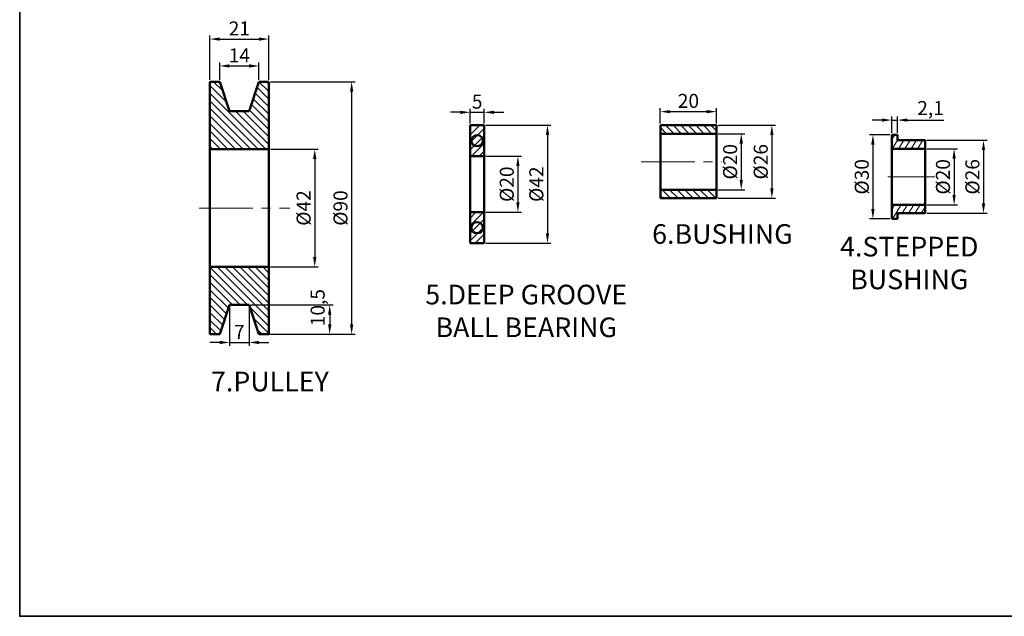
# Model space of a CAD drawing. Units: millimetres. Extents: x 54 to 669, y -108 to 325.
# Tile 1 of 3: x 54 to 404, y -108 to 104. Entities that reach past the tile are written whole.
import ezdxf

# ---------------------------------------------------------------- set-up
doc = ezdxf.new("R2010")
doc.units = ezdxf.units.MM
doc.linetypes.add('CENTER2', pattern=[28.575, 19.05, -3.175, 3.175, -3.175])
for name, color, linetype, lineweight in [('M-CNTR', 1, 'CENTER2', 18), ('M-DIMS', 2, 'Continuous', 25), ('M-HATC', 8, 'Continuous', 18), ('M-OUTL', 7, 'Continuous', 50), ('M-TEXT', 3, 'Continuous', 25), ('M-TTLB', 7, 'Continuous', 35)]:
    doc.layers.add(name, color=color, linetype=linetype, lineweight=lineweight)
doc.styles.get("Standard").update_dxf_attribs({"font": 'arial.ttf'})
doc.dimstyles.new('ISO-25', dxfattribs={"dimtxt": 5, "dimasz": 3.5, "dimexe": 1.25, "dimexo": 0.625, "dimtad": 1, "dimdec": 1, "dimtxsty": 'Standard', "dimcen": 2.5, "dimadec": 0, "dimazin": 0, "dimtfac": 1, "dimtdec": 1, "dimtmove": 0, "dimatfit": 3, "dimfxl": 1, "dimarcsym": 0})

# ---------------------------------------------------------------- blocks, each defined once
blk = doc.blocks.new('*U30')
at = {"layer": 'M-CNTR', "color": 0, "transparency": 16777216}
blk.add_line((-14.27, 0), (18.04, 0), dxfattribs=at)
blk = doc.blocks.new('*D31')
at = {"layer": 'Defpoints', "color": 0, "transparency": 16777216}
for p in [(138.84, 87.72), (124.84, 82.1), (138.84, 82.1)]:
    blk.add_point(p, dxfattribs=at)
at = {"layer": 'M-DIMS', "color": 0, "lineweight": -2, "transparency": 16777216}
for p, q in [((124.84, 82.72), (124.84, 88.97)), ((128.34, 87.72), (135.34, 87.72)), ((138.84, 82.72), (138.84, 88.97))]:
    blk.add_line(p, q, dxfattribs=at)
at = {"layer": 'M-DIMS', "color": 0, "transparency": 16777216}
for points in [[(128.34, 88.3), (128.34, 87.13), (124.84, 87.72)], [(135.34, 88.3), (135.34, 87.13), (138.84, 87.72)]]:
    blk.add_solid(points, dxfattribs=at)
at = {"layer": 'M-DIMS', "color": 0, "transparency": 16777216, "insert": (131.84, 90.85), "char_height": 5, "attachment_point": 5}
blk.add_mtext('14', dxfattribs=at)
blk = doc.blocks.new('*D32')
at = {"layer": 'Defpoints', "color": 0, "transparency": 16777216}
for p in [(142.34, 97.29), (121.34, 82.1), (142.34, 82.1)]:
    blk.add_point(p, dxfattribs=at)
at = {"layer": 'M-DIMS', "color": 0, "lineweight": -2, "transparency": 16777216}
for p, q in [((121.34, 82.72), (121.34, 98.54)), ((142.34, 82.72), (142.34, 98.54)), ((124.84, 97.29), (138.84, 97.29))]:
    blk.add_line(p, q, dxfattribs=at)
at = {"layer": 'M-DIMS', "color": 0, "transparency": 16777216}
for points in [[(124.84, 97.88), (124.84, 96.71), (121.34, 97.29)], [(138.84, 97.88), (138.84, 96.71), (142.34, 97.29)]]:
    blk.add_solid(points, dxfattribs=at)
at = {"layer": 'M-DIMS', "color": 0, "transparency": 16777216, "insert": (131.84, 100.43), "char_height": 5, "attachment_point": 5}
blk.add_mtext('21', dxfattribs=at)
blk = doc.blocks.new('*D33')
at = {"layer": 'Defpoints', "color": 0, "transparency": 16777216}
for p in [(142.34, 58.1), (142.34, 16.1), (158.7, 16.1)]:
    blk.add_point(p, dxfattribs=at)
at = {"layer": 'M-DIMS', "color": 0, "lineweight": -2, "transparency": 16777216}
for p, q in [((142.97, 58.1), (159.95, 58.1)), ((158.7, 54.6), (158.7, 19.6)), ((142.97, 16.1), (159.95, 16.1))]:
    blk.add_line(p, q, dxfattribs=at)
at = {"layer": 'M-DIMS', "color": 0, "transparency": 16777216}
for points in [[(158.11, 54.6), (159.28, 54.6), (158.7, 58.1)], [(158.11, 19.6), (159.28, 19.6), (158.7, 16.1)]]:
    blk.add_solid(points, dxfattribs=at)
at = {"layer": 'M-DIMS', "color": 0, "transparency": 16777216, "insert": (155.38, 37.1), "char_height": 5, "attachment_point": 5, "rotation": 90}
blk.add_mtext('%%C42', dxfattribs=at)
blk = doc.blocks.new('*D34')
at = {"layer": 'Defpoints', "color": 0, "transparency": 16777216}
for p in [(142.34, 82.1), (142.34, -7.9), (171.84, -7.9)]:
    blk.add_point(p, dxfattribs=at)
at = {"layer": 'M-DIMS', "color": 0, "lineweight": -2, "transparency": 16777216}
for p, q in [((142.97, 82.1), (173.09, 82.1)), ((171.84, 78.6), (171.84, -4.4)), ((142.97, -7.9), (173.09, -7.9))]:
    blk.add_line(p, q, dxfattribs=at)
at = {"layer": 'M-DIMS', "color": 0, "transparency": 16777216}
for points in [[(171.25, 78.6), (172.42, 78.6), (171.84, 82.1)], [(171.25, -4.4), (172.42, -4.4), (171.84, -7.9)]]:
    blk.add_solid(points, dxfattribs=at)
at = {"layer": 'M-DIMS', "color": 0, "transparency": 16777216, "insert": (168.52, 37.1), "char_height": 5, "attachment_point": 5, "rotation": 90}
blk.add_mtext('%%C90', dxfattribs=at)
blk = doc.blocks.new('*D35')
at = {"layer": 'Defpoints', "color": 0, "transparency": 16777216}
for p in [(135.34, 2.6), (138.84, -7.9), (164.02, -7.9)]:
    blk.add_point(p, dxfattribs=at)
at = {"layer": 'M-DIMS', "color": 0, "lineweight": -2, "transparency": 16777216}
for p, q in [((135.97, 2.6), (165.27, 2.6)), ((164.02, -0.9), (164.02, -4.4)), ((139.47, -7.9), (165.27, -7.9))]:
    blk.add_line(p, q, dxfattribs=at)
at = {"layer": 'M-DIMS', "color": 0, "transparency": 16777216}
for points in [[(163.44, -0.9), (164.61, -0.9), (164.02, 2.6)], [(163.44, -4.4), (164.61, -4.4), (164.02, -7.9)]]:
    blk.add_solid(points, dxfattribs=at)
at = {"layer": 'M-DIMS', "color": 0, "transparency": 16777216, "insert": (160.39, 1.61), "char_height": 5, "attachment_point": 5, "rotation": 90}
blk.add_mtext('10,5', dxfattribs=at)
blk = doc.blocks.new('*D36')
at = {"layer": 'Defpoints', "color": 0, "transparency": 16777216}
for p in [(128.34, 2.6), (135.34, 2.6), (135.34, -10.8)]:
    blk.add_point(p, dxfattribs=at)
at = {"layer": 'M-DIMS', "color": 0, "lineweight": -2, "transparency": 16777216}
for p, q in [((128.34, 1.97), (128.34, -12.05)), ((135.34, 1.97), (135.34, -12.05)), ((124.84, -10.8), (121.34, -10.8)), ((128.34, -10.8), (135.34, -10.8)), ((138.84, -10.8), (142.34, -10.8))]:
    blk.add_line(p, q, dxfattribs=at)
at = {"layer": 'M-DIMS', "color": 0, "transparency": 16777216}
for points in [[(124.84, -10.22), (124.84, -11.39), (128.34, -10.8)], [(138.84, -10.22), (138.84, -11.39), (135.34, -10.8)]]:
    blk.add_solid(points, dxfattribs=at)
at = {"layer": 'M-DIMS', "color": 0, "transparency": 16777216, "insert": (131.84, -7.68), "char_height": 5, "attachment_point": 5}
blk.add_mtext('7', dxfattribs=at)
blk = doc.blocks.new('*D40')
at = {"layer": 'Defpoints', "color": 0, "transparency": 16777216}
for p in [(219.04, 71.2), (214.04, 66.59), (219.04, 66.59)]:
    blk.add_point(p, dxfattribs=at)
at = {"layer": 'M-DIMS', "color": 0, "lineweight": -2, "transparency": 16777216}
for p, q in [((210.54, 71.2), (207.04, 71.2)), ((214.04, 67.21), (214.04, 72.45)), ((214.04, 71.2), (219.04, 71.2)), ((219.04, 67.21), (219.04, 72.45)), ((222.54, 71.2), (226.04, 71.2))]:
    blk.add_line(p, q, dxfattribs=at)
at = {"layer": 'M-DIMS', "color": 0, "transparency": 16777216}
for points in [[(210.54, 71.78), (210.54, 70.61), (214.04, 71.2)], [(222.54, 71.78), (222.54, 70.61), (219.04, 71.2)]]:
    blk.add_solid(points, dxfattribs=at)
at = {"layer": 'M-DIMS', "color": 0, "transparency": 16777216, "insert": (216.54, 74.36), "char_height": 5, "attachment_point": 5}
blk.add_mtext('5', dxfattribs=at)
blk = doc.blocks.new('*D41')
at = {"layer": 'Defpoints', "color": 0, "transparency": 16777216}
for p in [(219.04, 55.59), (219.04, 35.59), (231.05, 35.59)]:
    blk.add_point(p, dxfattribs=at)
at = {"layer": 'M-DIMS', "color": 0, "lineweight": -2, "transparency": 16777216}
for p, q in [((219.66, 55.59), (232.3, 55.59)), ((231.05, 52.09), (231.05, 39.09)), ((219.66, 35.59), (232.3, 35.59))]:
    blk.add_line(p, q, dxfattribs=at)
at = {"layer": 'M-DIMS', "color": 0, "transparency": 16777216}
for points in [[(230.47, 52.09), (231.63, 52.09), (231.05, 55.59)], [(230.47, 39.09), (231.63, 39.09), (231.05, 35.59)]]:
    blk.add_solid(points, dxfattribs=at)
at = {"layer": 'M-DIMS', "color": 0, "transparency": 16777216, "insert": (227.73, 45.59), "char_height": 5, "attachment_point": 5, "rotation": 90}
blk.add_mtext('%%C20', dxfattribs=at)
blk = doc.blocks.new('*D42')
at = {"layer": 'Defpoints', "color": 0, "transparency": 16777216}
for p in [(219.04, 66.59), (219.04, 24.59), (241.58, 24.59)]:
    blk.add_point(p, dxfattribs=at)
at = {"layer": 'M-DIMS', "color": 0, "lineweight": -2, "transparency": 16777216}
for p, q in [((219.66, 66.59), (242.83, 66.59)), ((241.58, 63.09), (241.58, 28.09)), ((219.66, 24.59), (242.83, 24.59))]:
    blk.add_line(p, q, dxfattribs=at)
at = {"layer": 'M-DIMS', "color": 0, "transparency": 16777216}
for points in [[(241, 63.09), (242.16, 63.09), (241.58, 66.59)], [(241, 28.09), (242.16, 28.09), (241.58, 24.59)]]:
    blk.add_solid(points, dxfattribs=at)
at = {"layer": 'M-DIMS', "color": 0, "transparency": 16777216, "insert": (238.26, 45.59), "char_height": 5, "width": 7.4511, "attachment_point": 5, "rotation": 90}
blk.add_mtext('%%C42', dxfattribs=at)
blk = doc.blocks.new('*U43')
at = {"layer": 'M-CNTR', "color": 0, "transparency": 16777216}
blk.add_line((-16.82, 0), (11.87, 0), dxfattribs=at)
blk = doc.blocks.new('*D44')
at = {"layer": 'Defpoints', "color": 0, "transparency": 16777216}
for p in [(301.77, 71.44), (281.77, 66.59), (301.77, 66.59)]:
    blk.add_point(p, dxfattribs=at)
at = {"layer": 'M-DIMS', "color": 0, "lineweight": -2, "transparency": 16777216}
for p, q in [((281.77, 67.21), (281.77, 72.69)), ((285.27, 71.44), (298.27, 71.44)), ((301.77, 67.21), (301.77, 72.69))]:
    blk.add_line(p, q, dxfattribs=at)
at = {"layer": 'M-DIMS', "color": 0, "transparency": 16777216}
for points in [[(285.27, 72.02), (285.27, 70.86), (281.77, 71.44)], [(298.27, 72.02), (298.27, 70.86), (301.77, 71.44)]]:
    blk.add_solid(points, dxfattribs=at)
at = {"layer": 'M-DIMS', "color": 0, "transparency": 16777216, "insert": (291.77, 74.62), "char_height": 5, "attachment_point": 5}
blk.add_mtext('20', dxfattribs=at)
blk = doc.blocks.new('*D45')
at = {"layer": 'Defpoints', "color": 0, "transparency": 16777216}
for p in [(301.77, 63.59), (301.77, 43.59), (310.59, 43.59)]:
    blk.add_point(p, dxfattribs=at)
at = {"layer": 'M-DIMS', "color": 0, "lineweight": -2, "transparency": 16777216}
for p, q in [((302.4, 63.59), (311.84, 63.59)), ((310.59, 60.09), (310.59, 47.09)), ((302.4, 43.59), (311.84, 43.59))]:
    blk.add_line(p, q, dxfattribs=at)
at = {"layer": 'M-DIMS', "color": 0, "transparency": 16777216}
for points in [[(310, 60.09), (311.17, 60.09), (310.59, 63.59)], [(310, 47.09), (311.17, 47.09), (310.59, 43.59)]]:
    blk.add_solid(points, dxfattribs=at)
at = {"layer": 'M-DIMS', "color": 0, "transparency": 16777216, "insert": (307.27, 53.59), "char_height": 5, "attachment_point": 5, "rotation": 90}
blk.add_mtext('%%C20', dxfattribs=at)
blk = doc.blocks.new('*D46')
at = {"layer": 'Defpoints', "color": 0, "transparency": 16777216}
for p in [(301.77, 66.59), (301.77, 40.59), (321.49, 40.59)]:
    blk.add_point(p, dxfattribs=at)
at = {"layer": 'M-DIMS', "color": 0, "lineweight": -2, "transparency": 16777216}
for p, q in [((302.4, 66.59), (322.74, 66.59)), ((321.49, 63.09), (321.49, 44.09)), ((302.4, 40.59), (322.74, 40.59))]:
    blk.add_line(p, q, dxfattribs=at)
at = {"layer": 'M-DIMS', "color": 0, "transparency": 16777216}
for points in [[(320.91, 63.09), (322.08, 63.09), (321.49, 66.59)], [(320.91, 44.09), (322.08, 44.09), (321.49, 40.59)]]:
    blk.add_solid(points, dxfattribs=at)
at = {"layer": 'M-DIMS', "color": 0, "transparency": 16777216, "insert": (318.17, 53.59), "char_height": 5, "attachment_point": 5, "rotation": 90}
blk.add_mtext('%%C26', dxfattribs=at)
blk = doc.blocks.new('*U52')
at = {"layer": 'M-CNTR', "color": 0, "transparency": 16777216}
blk.add_line((8.4, 0), (-8.4, 0), dxfattribs=at)
blk = doc.blocks.new('*D54')
at = {"layer": 'Defpoints', "color": 0, "transparency": 16777216}
for p in [(366.26, 68.44), (364.16, 63.22), (366.26, 63.22)]:
    blk.add_point(p, dxfattribs=at)
at = {"layer": 'M-DIMS', "color": 0, "lineweight": -2, "transparency": 16777216}
for p, q in [((360.66, 68.44), (357.16, 68.44)), ((364.16, 63.85), (364.16, 69.69)), ((364.16, 68.44), (366.26, 68.44)), ((366.26, 63.85), (366.26, 69.69)), ((369.76, 68.44), (382.73, 68.44))]:
    blk.add_line(p, q, dxfattribs=at)
at = {"layer": 'M-DIMS', "color": 0, "transparency": 16777216}
for points in [[(360.66, 69.02), (360.66, 67.85), (364.16, 68.44)], [(369.76, 69.02), (369.76, 67.85), (366.26, 68.44)]]:
    blk.add_solid(points, dxfattribs=at)
at = {"layer": 'M-DIMS', "color": 0, "transparency": 16777216, "insert": (378, 72.07), "char_height": 5, "attachment_point": 5}
blk.add_mtext('2,1', dxfattribs=at)
blk = doc.blocks.new('*D55')
at = {"layer": 'Defpoints', "color": 0, "transparency": 16777216}
for p in [(376.06, 58.22), (376.06, 38.22), (386.39, 38.22)]:
    blk.add_point(p, dxfattribs=at)
at = {"layer": 'M-DIMS', "color": 0, "lineweight": -2, "transparency": 16777216}
for p, q in [((376.68, 58.22), (387.64, 58.22)), ((386.39, 54.72), (386.39, 41.72)), ((376.68, 38.22), (387.64, 38.22))]:
    blk.add_line(p, q, dxfattribs=at)
at = {"layer": 'M-DIMS', "color": 0, "transparency": 16777216}
for points in [[(385.81, 54.72), (386.97, 54.72), (386.39, 58.22)], [(385.81, 41.72), (386.97, 41.72), (386.39, 38.22)]]:
    blk.add_solid(points, dxfattribs=at)
at = {"layer": 'M-DIMS', "color": 0, "transparency": 16777216, "insert": (383.07, 48.22), "char_height": 5, "width": 7.4852, "attachment_point": 5, "rotation": 90}
blk.add_mtext('%%C20', dxfattribs=at)
blk = doc.blocks.new('*D56')
at = {"layer": 'Defpoints', "color": 0, "transparency": 16777216}
for p in [(376.06, 61.22), (376.06, 35.22), (396.86, 35.22)]:
    blk.add_point(p, dxfattribs=at)
at = {"layer": 'M-DIMS', "color": 0, "lineweight": -2, "transparency": 16777216}
for p, q in [((376.68, 61.22), (398.11, 61.22)), ((396.86, 57.72), (396.86, 38.72)), ((376.68, 35.22), (398.11, 35.22))]:
    blk.add_line(p, q, dxfattribs=at)
at = {"layer": 'M-DIMS', "color": 0, "transparency": 16777216}
for points in [[(396.28, 57.72), (397.45, 57.72), (396.86, 61.22)], [(396.28, 38.72), (397.45, 38.72), (396.86, 35.22)]]:
    blk.add_solid(points, dxfattribs=at)
at = {"layer": 'M-DIMS', "color": 0, "transparency": 16777216, "insert": (393.55, 48.22), "char_height": 5, "attachment_point": 5, "rotation": 90}
blk.add_mtext('%%C26', dxfattribs=at)
blk = doc.blocks.new('*D57')
at = {"layer": 'Defpoints', "color": 0, "transparency": 16777216}
for p in [(364.16, 63.22), (357.47, 33.22), (364.16, 33.22)]:
    blk.add_point(p, dxfattribs=at)
at = {"layer": 'M-DIMS', "color": 0, "lineweight": -2, "transparency": 16777216}
for p, q in [((363.53, 63.22), (356.22, 63.22)), ((357.47, 59.72), (357.47, 36.72)), ((363.53, 33.22), (356.22, 33.22))]:
    blk.add_line(p, q, dxfattribs=at)
at = {"layer": 'M-DIMS', "color": 0, "transparency": 16777216}
for points in [[(356.89, 59.72), (358.06, 59.72), (357.47, 63.22)], [(356.89, 36.72), (358.06, 36.72), (357.47, 33.22)]]:
    blk.add_solid(points, dxfattribs=at)
at = {"layer": 'M-DIMS', "color": 0, "transparency": 16777216, "insert": (354.16, 48.22), "char_height": 5, "attachment_point": 5, "rotation": 90}
blk.add_mtext('%%C30', dxfattribs=at)

msp = doc.modelspace()

# ---------------------------------------------------------------- hatches: boundary and pattern name
at = {"layer": 'M-HATC'}
h = msp.add_hatch(dxfattribs=at)
h.set_pattern_fill('ANSI31', color=256, scale=0.6, angle=90)
h.paths.add_polyline_path([(142.3403, 82.0968), (138.8403, 82.0968), (135.3403, 71.5968), (128.3403, 71.5968), (124.8403, 82.0968), (121.3403, 82.0968), (121.3403, 58.0968), (142.3403, 58.0968)])
h.paths.add_polyline_path([(142.3403, 16.0968), (121.3403, 16.0968), (121.3403, -7.9032), (124.8403, -7.9032), (128.3403, 2.5968), (135.3403, 2.5968), (138.8403, -7.9032), (142.3403, -7.9032)])
h = msp.add_hatch(dxfattribs=at)
h.set_pattern_fill('ANSI31', color=256, scale=0.6)
h.paths.add_polyline_path([(219.0393, 66.5889), (214.0393, 66.5889), (214.0393, 55.5889), (219.0393, 55.5889)])
h.paths.add_polyline_path([(219.0393, 35.5889), (214.0393, 35.5889), (214.0393, 24.5889), (219.0393, 24.5889)])
h = msp.add_hatch(dxfattribs=at)
h.set_pattern_fill('ANSI31', color=256, scale=0.6, angle=90)
h.paths.add_polyline_path([(301.7726, 66.5889), (281.7726, 66.5889), (281.7726, 63.5889), (301.7726, 63.5889)])
h.paths.add_polyline_path([(301.7726, 43.5889), (281.7726, 43.5889), (281.7726, 40.5889), (301.7726, 40.5889)])
h = msp.add_hatch(dxfattribs=at)
h.set_pattern_fill('ANSI31', color=256, scale=0.6, angle=13)
h.paths.add_polyline_path([(376.0586, 61.2211), (366.2586, 61.2211), (366.2586, 63.2211), (364.1586, 63.2211), (364.1586, 58.2211), (376.0586, 58.2211)])
h.paths.add_polyline_path([(376.0586, 38.2211), (364.1586, 38.2211), (364.1586, 33.2211), (366.2586, 33.2211), (366.2586, 35.2211), (376.0586, 35.2211)])

# ---------------------------------------------------------------- linework, layer by layer
at = {"layer": 'M-OUTL'}
for p, q in [((121.3403, 82.0968), (124.8403, 82.0968)), ((121.3403, -7.9032), (121.3403, 82.0968)), ((124.8403, 82.0968), (121.3403, 82.0968)), ((124.8403, 82.0968), (128.3403, 71.5968)), ((138.8403, 82.0968), (135.3403, 71.5968)), ((142.3403, 82.0968), (138.8403, 82.0968)), ((138.8403, 82.0968), (142.3403, 82.0968)), ((142.3403, 82.0968), (142.3403, -7.9032)), ((135.3403, 71.5968), (128.3403, 71.5968)), ((214.0393, 66.5889), (214.0393, 24.5889)), ((219.0393, 66.5889), (214.0393, 66.5889)), ((219.0393, 24.5889), (219.0393, 66.5889)), ((281.7726, 66.5889), (301.7726, 66.5889)), ((281.7726, 40.5889), (281.7726, 66.5889)), ((301.7726, 63.5889), (281.7726, 63.5889)), ((301.7726, 66.5889), (301.7726, 40.5889)), ((364.1586, 63.2211), (364.1586, 33.2211)), ((366.2586, 63.2211), (364.1586, 63.2211)), ((366.2586, 61.2211), (366.2586, 63.2211)), ((376.0586, 61.2211), (366.2586, 61.2211)), ((376.0586, 35.2211), (376.0586, 61.2211)), ((142.3403, 58.0968), (121.3403, 58.0968)), ((376.0586, 58.2211), (364.1586, 58.2211)), ((219.0393, 55.5889), (214.0393, 55.5889)), ((301.7726, 43.5889), (281.7726, 43.5889)), ((301.7726, 40.5889), (281.7726, 40.5889)), ((219.0393, 35.5889), (214.0393, 35.5889)), ((376.0586, 38.2211), (364.1586, 38.2211)), ((366.2586, 33.2211), (366.2586, 35.2211)), ((366.2586, 35.2211), (376.0586, 35.2211)), ((364.1586, 33.2211), (366.2586, 33.2211)), ((214.0393, 24.5889), (219.0393, 24.5889)), ((142.3403, 16.0968), (121.3403, 16.0968)), ((124.8403, -7.9032), (128.3403, 2.5968)), ((135.3403, 2.5968), (128.3403, 2.5968)), ((138.8403, -7.9032), (135.3403, 2.5968)), ((124.8403, -7.9032), (121.3403, -7.9032)), ((142.3403, -7.9032), (138.8403, -7.9032))]:
    msp.add_line(p, q, dxfattribs=at)
for centre in [(216.5393, 61.0889), (216.5393, 30.0889)]:
    msp.add_circle(centre, 2, dxfattribs=at)
at = {"layer": 'M-TTLB'}
msp.add_lwpolyline([(53.6241, 324.969), (668.8363, 324.969), (668.8363, -108.3789), (53.6241, -108.3789)], close=True, dxfattribs=at)

# ---------------------------------------------------------------- block references
at = {"layer": 'M-CNTR'}
for name, p in [('*U43', (291.7726, 53.5889)), ('*U52', (371.1586, 48.2211)), ('*U30', (131.8403, 37.0968))]:
    msp.add_blockref(name, p, dxfattribs=at)

# ---------------------------------------------------------------- texts
at = {"layer": 'M-TEXT', "char_height": 7, "attachment_point": 1}
for s, width, insert in [('6.BUSHING', 45.804463, (278.856, 31.3434)), ('\\pxqc;4.STEPPED BUSHING', 45.804463, (347.5224, 26.8426)), ('\\pxqc;5.DEEP GROOVE BALL BEARING', 90.278815, (188.8739, 9.7664)), ('7.PULLEY', 45.804463, (121.7507, -21.2176))]:
    msp.add_mtext_dynamic_manual_height_columns(s, width=width, gutter_width=12.5, heights=[0], dxfattribs=dict(at, insert=insert))

# ---------------------------------------------------------------- dimensions: what is measured, and where the dimension line sits
at = {"layer": 'M-DIMS'}
for base, p1, p2, picture, middle in [((142.3403, 97.2934), (121.3403, 82.0968), (142.3403, 82.0968), '*D32', (131.8403, 100.4286)), ((138.8403, 87.7157), (124.8403, 82.0968), (138.8403, 82.0968), '*D31', (131.8403, 90.851)), ((219.0393, 71.1965), (214.0393, 66.5889), (219.0393, 66.5889), '*D40', (216.5393, 74.3641)), ((301.7726, 71.4413), (281.7726, 66.5889), (301.7726, 66.5889), '*D44', (291.7726, 74.6192)), ((366.2586, 68.437), (364.1586, 63.2211), (366.2586, 63.2211), '*D54', (377.9952, 72.0668)), ((135.3403, -10.8038), (128.3403, 2.5968), (135.3403, 2.5968), '*D36', (131.8403, -7.6788))]:
    dim = msp.add_linear_dim(base=base, p1=p1, p2=p2, dimstyle='ISO-25', override={"dimclrd": 0, "dimclre": 0, "dimclrt": 0}, dxfattribs=at)
    dim.commit()
    dim.dimension.update_dxf_attribs({"geometry": picture, "text_midpoint": middle})
for base, p1, p2, picture, middle in [((171.8354, -7.9032), (142.3403, 82.0968), (142.3403, -7.9032), '*D34', (168.5177, 37.0968)), ((241.5805, 24.5889), (219.0393, 66.5889), (219.0393, 24.5889), '*D42', (238.2628, 45.5889)), ((321.4923, 40.5889), (301.7726, 66.5889), (301.7726, 40.5889), '*D46', (318.1746, 53.5889)), ((310.5879, 43.5889), (301.7726, 63.5889), (301.7726, 43.5889), '*D45', (307.2702, 53.5889)), ((357.4741, 33.2211), (364.1586, 63.2211), (364.1586, 33.2211), '*D57', (354.1564, 48.2211)), ((396.865, 35.2211), (376.0586, 61.2211), (376.0586, 35.2211), '*D56', (393.5473, 48.2211)), ((158.6977, 16.0968), (142.3403, 58.0968), (142.3403, 16.0968), '*D33', (155.38, 37.0968)), ((386.3902, 38.2211), (376.0586, 58.2211), (376.0586, 38.2211), '*D55', (383.0725, 48.2211)), ((231.0498, 35.5889), (219.0393, 55.5889), (219.0393, 35.5889), '*D41', (227.7321, 45.5889))]:
    dim = msp.add_linear_dim(base=base, p1=p1, p2=p2, angle=90, text='%%C<>', dimstyle='ISO-25', override={"dimclrd": 0, "dimclre": 0, "dimclrt": 0}, dxfattribs=at)
    dim.commit()
    dim.dimension.update_dxf_attribs({"geometry": picture, "text_midpoint": middle})
dim = msp.add_linear_dim(base=(164.0247, -7.9032), p1=(135.3403, 2.5968), p2=(138.8403, -7.9032), angle=90, dimstyle='ISO-25', override={"dimclrd": 0, "dimclre": 0, "dimclrt": 0}, dxfattribs=at)
dim.commit()
dim.dimension.update_dxf_attribs({"geometry": '*D35', "text_midpoint": (164.0247, 1.6086), "dimtype": 160})

doc.saveas('drawing.dxf')
